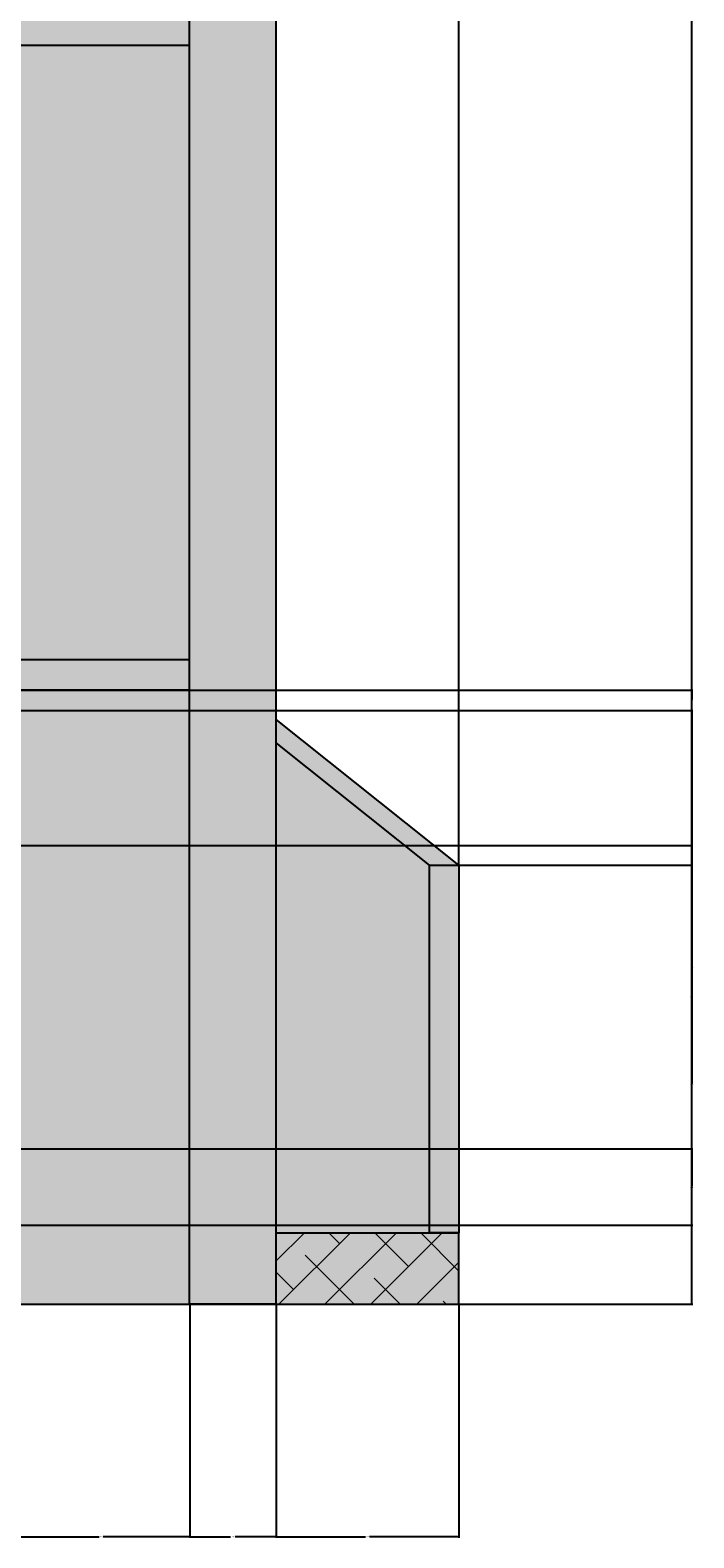
# Model space of a CAD drawing. Units: inches. Extents: x 3024 to 4744, y 1110 to 2100.
# Tile 16 of 29: x 3657 to 3787, y 1110 to 1405. Entities that reach past the tile are written whole.
import ezdxf

# ---------------------------------------------------------------- set-up
doc = ezdxf.new("R2010")
doc.units = ezdxf.units.IN
for name, color, linetype, lineweight in [('A-ANNO-DIMS', 2, 'Continuous', 18), ('A-ELEV', 7, 'Continuous', 25), ('A-ELEV-PATT', 252, 'Continuous', 13)]:
    doc.layers.add(name, color=color, linetype=linetype, lineweight=lineweight)
doc.styles.get("Standard").update_dxf_attribs({"font": 'arial.ttf'})
doc.dimstyles.get("Standard").update_dxf_attribs({"dimtxt": 0.18, "dimasz": 0.18, "dimexe": 0.18, "dimexo": 0.0625, "dimgap": 0.09, "dimtad": 0, "dimtih": 1, "dimtoh": 1, "dimdec": 1, "dimzin": 0, "dimdsep": 46, "dimlunit": 3, "dimtxsty": 'Standard', "dimcen": 0.09, "dimadec": 0, "dimazin": 0, "dimtfac": 1, "dimtdec": 1, "dimtofl": 0, "dimtmove": 0, "dimatfit": 3, "dimfxl": 1, "dimtolj": 1, "dimtzin": 0, "dimarcsym": 0})

# ---------------------------------------------------------------- blocks, each defined once
blk = doc.blocks.new('*D61')
at = {"layer": 'A-ANNO-DIMS', "color": 0, "lineweight": -2, "transparency": 16777216}
for p, q in [((3654.04, 1155.55), (3654.04, 1109.93)), ((3688.56, 1155.55), (3688.56, 1109.93)), ((3654.22, 1110.11), (3670.91, 1110.11)), ((3688.38, 1110.11), (3671.69, 1110.11))]:
    blk.add_line(p, q, dxfattribs=at)
at = {"layer": 'A-ANNO-DIMS', "color": 0, "transparency": 16777216}
for points in [[(3654.22, 1110.14), (3654.22, 1110.08), (3654.04, 1110.11)], [(3688.38, 1110.14), (3688.38, 1110.08), (3688.56, 1110.11)]]:
    blk.add_solid(points, dxfattribs=at)
at = {"layer": 'Defpoints', "color": 0, "transparency": 16777216}
for p in [(3654.04, 1155.61), (3688.56, 1155.61), (3688.56, 1110.11)]:
    blk.add_point(p, dxfattribs=at)
at = {"layer": 'A-ANNO-DIMS', "color": 0, "transparency": 16777216, "insert": (3671.3, 1110.11), "char_height": 0.18, "attachment_point": 5}
blk.add_mtext('\\A1;34.52', dxfattribs=at)
blk = doc.blocks.new('*D62')
at = {"layer": 'A-ANNO-DIMS', "color": 0, "lineweight": -2, "transparency": 16777216}
for p, q in [((3688.56, 1155.55), (3688.56, 1109.93)), ((3705.47, 1155.55), (3705.47, 1109.93)), ((3688.74, 1110.11), (3696.56, 1110.11)), ((3705.29, 1110.11), (3697.47, 1110.11))]:
    blk.add_line(p, q, dxfattribs=at)
at = {"layer": 'A-ANNO-DIMS', "color": 0, "transparency": 16777216}
for points in [[(3688.74, 1110.14), (3688.74, 1110.08), (3688.56, 1110.11)], [(3705.29, 1110.14), (3705.29, 1110.08), (3705.47, 1110.11)]]:
    blk.add_solid(points, dxfattribs=at)
at = {"layer": 'Defpoints', "color": 0, "transparency": 16777216}
for p in [(3688.56, 1155.61), (3705.47, 1155.61), (3705.47, 1110.11)]:
    blk.add_point(p, dxfattribs=at)
at = {"layer": 'A-ANNO-DIMS', "color": 0, "transparency": 16777216, "insert": (3697.02, 1110.11), "char_height": 0.18, "attachment_point": 5}
blk.add_mtext('\\A1;16.913', dxfattribs=at)
blk = doc.blocks.new('*D63')
at = {"layer": 'A-ANNO-DIMS', "color": 0, "lineweight": -2, "transparency": 16777216}
for p, q in [((3705.47, 1155.55), (3705.47, 1109.93)), ((3741.15, 1155.55), (3741.15, 1109.93)), ((3705.65, 1110.11), (3722.92, 1110.11)), ((3740.97, 1110.11), (3723.71, 1110.11))]:
    blk.add_line(p, q, dxfattribs=at)
at = {"layer": 'A-ANNO-DIMS', "color": 0, "transparency": 16777216}
for points in [[(3705.65, 1110.14), (3705.65, 1110.08), (3705.47, 1110.11)], [(3740.97, 1110.14), (3740.97, 1110.08), (3741.15, 1110.11)]]:
    blk.add_solid(points, dxfattribs=at)
at = {"layer": 'Defpoints', "color": 0, "transparency": 16777216}
for p in [(3705.47, 1155.61), (3741.15, 1155.61), (3741.15, 1110.11)]:
    blk.add_point(p, dxfattribs=at)
at = {"layer": 'A-ANNO-DIMS', "color": 0, "transparency": 16777216, "insert": (3723.31, 1110.11), "char_height": 0.18, "attachment_point": 5}
blk.add_mtext('\\A1;35.68', dxfattribs=at)
blk = doc.blocks.new('*D64')
at = {"layer": 'A-ANNO-DIMS', "color": 0, "lineweight": -2, "transparency": 16777216}
for p, q in [((3069.79, 1241.5), (3069.79, 2100.44)), ((3069.97, 2100.26), (3405.08, 2100.26)), ((3740.97, 2100.26), (3405.87, 2100.26)), ((3741.15, 1241.5), (3741.15, 2100.44))]:
    blk.add_line(p, q, dxfattribs=at)
at = {"layer": 'A-ANNO-DIMS', "color": 0, "transparency": 16777216}
for points in [[(3069.97, 2100.29), (3069.97, 2100.23), (3069.79, 2100.26)], [(3740.97, 2100.29), (3740.97, 2100.23), (3741.15, 2100.26)]]:
    blk.add_solid(points, dxfattribs=at)
at = {"layer": 'Defpoints', "color": 0, "transparency": 16777216}
for p in [(3741.15, 2100.26), (3069.79, 1241.43), (3741.15, 1241.43)]:
    blk.add_point(p, dxfattribs=at)
at = {"layer": 'A-ANNO-DIMS', "color": 0, "transparency": 16777216, "insert": (3405.47, 2100.26), "char_height": 0.18, "attachment_point": 5}
blk.add_mtext('\\A1;671.4', dxfattribs=at)
blk = doc.blocks.new('*D75')
at = {"layer": 'A-ANNO-DIMS', "color": 0, "lineweight": -2, "transparency": 16777216}
for p, q in [((3491.89, 2054.76), (3786.83, 2054.76)), ((3786.65, 2054.58), (3786.65, 1605.37)), ((3786.65, 1155.79), (3786.65, 1605)), ((3741.21, 1155.61), (3786.83, 1155.61))]:
    blk.add_line(p, q, dxfattribs=at)
at = {"layer": 'A-ANNO-DIMS', "color": 0, "transparency": 16777216}
for points in [[(3786.62, 2054.58), (3786.68, 2054.58), (3786.65, 2054.76)], [(3786.62, 1155.79), (3786.68, 1155.79), (3786.65, 1155.61)]]:
    blk.add_solid(points, dxfattribs=at)
at = {"layer": 'Defpoints', "color": 0, "transparency": 16777216}
for p in [(3491.83, 2054.76), (3786.65, 2054.76), (3741.15, 1155.61)]:
    blk.add_point(p, dxfattribs=at)
at = {"layer": 'A-ANNO-DIMS', "color": 0, "transparency": 16777216, "insert": (3786.65, 1605.18), "char_height": 0.18, "attachment_point": 5}
blk.add_mtext('\\A1;899.1', dxfattribs=at)
blk = doc.blocks.new('*D79')
at = {"layer": 'A-ANNO-DIMS', "color": 0, "lineweight": -2, "transparency": 16777216}
for p, q in [((3741.21, 1241.43), (3786.83, 1241.43)), ((3786.65, 1241.25), (3786.65, 1198.7)), ((3786.65, 1155.79), (3786.65, 1198.34)), ((3741.21, 1155.61), (3786.83, 1155.61))]:
    blk.add_line(p, q, dxfattribs=at)
at = {"layer": 'A-ANNO-DIMS', "color": 0, "transparency": 16777216}
for points in [[(3786.62, 1241.25), (3786.68, 1241.25), (3786.65, 1241.43)], [(3786.62, 1155.79), (3786.68, 1155.79), (3786.65, 1155.61)]]:
    blk.add_solid(points, dxfattribs=at)
at = {"layer": 'Defpoints', "color": 0, "transparency": 16777216}
for p in [(3741.15, 1241.43), (3786.65, 1241.43), (3741.15, 1155.61)]:
    blk.add_point(p, dxfattribs=at)
at = {"layer": 'A-ANNO-DIMS', "color": 0, "transparency": 16777216, "insert": (3786.65, 1198.52), "char_height": 0.18, "attachment_point": 5}
blk.add_mtext('\\A1;85.82', dxfattribs=at)
blk = doc.blocks.new('*D120')
at = {"layer": 'A-ANNO-DIMS', "color": 0, "lineweight": -2, "transparency": 16777216}
for p, q in [((3270.45, 1271.61), (3786.83, 1271.61)), ((3786.65, 1271.43), (3786.65, 1221.5)), ((3786.65, 1171.2), (3786.65, 1221.14)), ((3274.45, 1171.02), (3786.83, 1171.02))]:
    blk.add_line(p, q, dxfattribs=at)
at = {"layer": 'A-ANNO-DIMS', "color": 0, "transparency": 16777216}
for points in [[(3786.62, 1271.43), (3786.68, 1271.43), (3786.65, 1271.61)], [(3786.62, 1171.2), (3786.68, 1171.2), (3786.65, 1171.02)]]:
    blk.add_solid(points, dxfattribs=at)
at = {"layer": 'Defpoints', "color": 0, "transparency": 16777216}
for p in [(3270.39, 1271.61), (3786.65, 1271.61), (3274.39, 1171.02)]:
    blk.add_point(p, dxfattribs=at)
at = {"layer": 'A-ANNO-DIMS', "color": 0, "transparency": 16777216, "insert": (3786.65, 1221.32), "char_height": 0.18, "attachment_point": 5}
blk.add_mtext('\\A1;100.59', dxfattribs=at)
blk = doc.blocks.new('*D121')
at = {"layer": 'A-ANNO-DIMS', "color": 0, "lineweight": -2, "transparency": 16777216}
for p, q in [((3274.45, 1275.61), (3786.83, 1275.61)), ((3786.65, 1275.43), (3786.65, 1273.79)), ((3786.65, 1271.79), (3786.65, 1273.43)), ((3270.45, 1271.61), (3786.83, 1271.61))]:
    blk.add_line(p, q, dxfattribs=at)
at = {"layer": 'A-ANNO-DIMS', "color": 0, "transparency": 16777216}
for points in [[(3786.62, 1275.43), (3786.68, 1275.43), (3786.65, 1275.61)], [(3786.62, 1271.79), (3786.68, 1271.79), (3786.65, 1271.61)]]:
    blk.add_solid(points, dxfattribs=at)
at = {"layer": 'Defpoints', "color": 0, "transparency": 16777216}
for p in [(3274.39, 1275.61), (3786.65, 1275.61), (3270.39, 1271.61)]:
    blk.add_point(p, dxfattribs=at)
at = {"layer": 'A-ANNO-DIMS', "color": 0, "transparency": 16777216, "insert": (3786.65, 1273.61), "char_height": 0.18, "attachment_point": 5}
blk.add_mtext('\\A1;4.00', dxfattribs=at)
blk = doc.blocks.new('*D122')
at = {"layer": 'A-ANNO-DIMS', "color": 0, "lineweight": -2, "transparency": 16777216}
for p, q in [((3228.45, 1185.95), (3786.83, 1185.95)), ((3786.65, 1185.77), (3786.65, 1178.67)), ((3786.65, 1171.2), (3786.65, 1178.31)), ((3270.45, 1171.02), (3786.83, 1171.02))]:
    blk.add_line(p, q, dxfattribs=at)
at = {"layer": 'A-ANNO-DIMS', "color": 0, "transparency": 16777216}
for points in [[(3786.62, 1185.77), (3786.68, 1185.77), (3786.65, 1185.95)], [(3786.62, 1171.2), (3786.68, 1171.2), (3786.65, 1171.02)]]:
    blk.add_solid(points, dxfattribs=at)
at = {"layer": 'Defpoints', "color": 0, "transparency": 16777216}
for p in [(3228.39, 1185.95), (3270.39, 1171.02), (3786.65, 1171.02)]:
    blk.add_point(p, dxfattribs=at)
at = {"layer": 'A-ANNO-DIMS', "color": 0, "transparency": 16777216, "insert": (3786.65, 1178.49), "char_height": 0.18, "attachment_point": 5}
blk.add_mtext('\\A1;14.928', dxfattribs=at)
blk = doc.blocks.new('*D123')
at = {"layer": 'A-ANNO-DIMS', "color": 0, "lineweight": -2, "transparency": 16777216}
for p, q in [((3228.45, 1245.27), (3786.83, 1245.27)), ((3786.65, 1245.09), (3786.65, 1215.79)), ((3786.65, 1186.13), (3786.65, 1215.43)), ((3228.45, 1185.95), (3786.83, 1185.95))]:
    blk.add_line(p, q, dxfattribs=at)
at = {"layer": 'A-ANNO-DIMS', "color": 0, "transparency": 16777216}
for points in [[(3786.62, 1245.09), (3786.68, 1245.09), (3786.65, 1245.27)], [(3786.62, 1186.13), (3786.68, 1186.13), (3786.65, 1185.95)]]:
    blk.add_solid(points, dxfattribs=at)
at = {"layer": 'Defpoints', "color": 0, "transparency": 16777216}
for p in [(3228.39, 1245.27), (3786.65, 1245.27), (3228.39, 1185.95)]:
    blk.add_point(p, dxfattribs=at)
at = {"layer": 'A-ANNO-DIMS', "color": 0, "transparency": 16777216, "insert": (3786.65, 1215.61), "char_height": 0.18, "attachment_point": 5}
blk.add_mtext('\\A1;59.32', dxfattribs=at)

msp = doc.modelspace()

# ---------------------------------------------------------------- hatches: boundary and pattern name
at = {"layer": 'A-ELEV-PATT'}
h = msp.add_hatch(color=256, dxfattribs=at)
h.dxf.hatch_style = 1
h.paths.add_polyline_path([(3705.4722, 2014.6567), (3688.5588, 2014.6567), (3481.2411, 2014.6567), (3481.2411, 2009.1664), (3688.5588, 2009.1664), (3688.5588, 1155.6112), (3705.4722, 1155.6112), (3705.4722, 1911.6112)])
h = msp.add_hatch(color=256, dxfattribs=at)
h.dxf.hatch_style = 1
h.paths.add_polyline_path([(3154.3287, 1897.4879), (3148.9694, 1897.4879), (3148.9694, 1905.6112), (3105.4722, 1905.6112), (3105.4722, 1785.6112), (3148.9694, 1785.6112), (3148.9694, 1795.0431), (3151.6604, 1795.0431), (3151.6604, 1806.8674), (3154.3287, 1806.8674)])
h.paths.add_polyline_path([(3329.7033, 1905.6112), (3292.6051, 1905.6112), (3292.6051, 1897.4879), (3287.2458, 1897.4879), (3287.2458, 1806.8674), (3288.3759, 1806.8674), (3288.3759, 1795.0431), (3292.6051, 1795.0431), (3292.6051, 1785.6112), (3329.7033, 1785.6112)])
h.paths.add_polyline_path([(3154.3287, 1771.4879), (3148.9694, 1771.4879), (3148.9694, 1779.6112), (3105.4722, 1779.6112), (3105.4722, 1659.6112), (3148.9694, 1659.6112), (3148.9694, 1669.0431), (3151.6604, 1669.0431), (3151.6604, 1680.8674), (3154.3287, 1680.8674)])
h.paths.add_polyline_path([(3329.7033, 1779.6112), (3292.6051, 1779.6112), (3292.6051, 1771.4879), (3287.2458, 1771.4879), (3287.2458, 1680.8674), (3288.3759, 1680.8674), (3288.3759, 1669.0431), (3292.6051, 1669.0431), (3292.6051, 1659.6112), (3329.7033, 1659.6112)])
h.paths.add_polyline_path([(3154.3287, 1645.4879), (3148.9694, 1645.4879), (3148.9694, 1653.6112), (3105.4722, 1653.6112), (3105.4722, 1533.6112), (3148.9694, 1533.6112), (3148.9694, 1543.0431), (3151.6604, 1543.0431), (3151.6604, 1554.8674), (3154.3287, 1554.8674)])
h.paths.add_polyline_path([(3329.7033, 1653.6112), (3292.6051, 1653.6112), (3292.6051, 1645.4879), (3287.2458, 1645.4879), (3287.2458, 1554.8674), (3288.3759, 1554.8674), (3288.3759, 1543.0431), (3292.6051, 1543.0431), (3292.6051, 1533.6112), (3329.7033, 1533.6112)])
h.paths.add_polyline_path([(3329.7033, 1527.6112), (3292.6051, 1527.6112), (3292.6051, 1519.4879), (3287.2458, 1519.4879), (3287.2458, 1428.8674), (3288.3759, 1428.8674), (3288.3759, 1417.0431), (3292.6051, 1417.0431), (3292.6051, 1407.6112), (3329.7033, 1407.6112)])
h.paths.add_polyline_path([(3329.7033, 1401.6112), (3292.6051, 1401.6112), (3292.6051, 1393.4879), (3287.2458, 1393.4879), (3287.2458, 1302.8674), (3288.3759, 1302.8674), (3288.3759, 1291.0431), (3292.6051, 1291.0431), (3292.6051, 1281.6112), (3329.7033, 1281.6112)])
h.paths.add_polyline_path([(3154.3287, 1393.4879), (3148.9694, 1393.4879), (3148.9694, 1401.6112), (3105.4722, 1401.6112), (3105.4722, 1281.6112), (3148.9694, 1281.6112), (3148.9694, 1291.0431), (3151.6604, 1291.0431), (3151.6604, 1302.8674), (3154.3287, 1302.8674)])
h.paths.add_polyline_path([(3154.3287, 1519.4879), (3148.9694, 1519.4879), (3148.9694, 1527.6112), (3105.4722, 1527.6112), (3105.4722, 1407.6112), (3148.9694, 1407.6112), (3148.9694, 1417.0431), (3151.6604, 1417.0431), (3151.6604, 1428.8674), (3154.3287, 1428.8674)])
h.paths.add_polyline_path([(3515.7606, 1897.4879), (3510.4013, 1897.4879), (3510.4013, 1905.6112), (3481.2411, 1905.6112), (3481.2411, 1785.6112), (3510.4013, 1785.6112), (3510.4013, 1795.0431), (3513.0923, 1795.0431), (3513.0923, 1806.8674), (3515.7606, 1806.8674)])
h.paths.add_polyline_path([(3688.5588, 1905.6112), (3654.037, 1905.6112), (3654.037, 1897.4879), (3648.6777, 1897.4879), (3648.6777, 1806.8674), (3649.8078, 1806.8674), (3649.8078, 1795.0431), (3654.037, 1795.0431), (3654.037, 1785.6112), (3688.5588, 1785.6112)])
h.paths.add_polyline_path([(3515.7606, 1771.4879), (3510.4013, 1771.4879), (3510.4013, 1779.6112), (3481.2411, 1779.6112), (3481.2411, 1659.6112), (3510.4013, 1659.6112), (3510.4013, 1669.0431), (3513.0923, 1669.0431), (3513.0923, 1680.8674), (3515.7606, 1680.8674)])
h.paths.add_polyline_path([(3688.5588, 1779.6112), (3654.037, 1779.6112), (3654.037, 1771.4879), (3648.6777, 1771.4879), (3648.6777, 1680.8674), (3649.8078, 1680.8674), (3649.8078, 1669.0431), (3654.037, 1669.0431), (3654.037, 1659.6112), (3688.5588, 1659.6112)])
h.paths.add_polyline_path([(3515.7606, 1645.4879), (3510.4013, 1645.4879), (3510.4013, 1653.6112), (3481.2411, 1653.6112), (3481.2411, 1533.6112), (3510.4013, 1533.6112), (3510.4013, 1543.0431), (3513.0923, 1543.0431), (3513.0923, 1554.8674), (3515.7606, 1554.8674)])
h.paths.add_polyline_path([(3688.5588, 1653.6112), (3654.037, 1653.6112), (3654.037, 1645.4879), (3648.6777, 1645.4879), (3648.6777, 1554.8674), (3649.8078, 1554.8674), (3649.8078, 1543.0431), (3654.037, 1543.0431), (3654.037, 1533.6112), (3688.5588, 1533.6112)])
h.paths.add_polyline_path([(3515.7606, 1519.4879), (3510.4013, 1519.4879), (3510.4013, 1527.6112), (3481.2411, 1527.6112), (3481.2411, 1407.6112), (3510.4013, 1407.6112), (3510.4013, 1417.0431), (3513.0923, 1417.0431), (3513.0923, 1428.8674), (3515.7606, 1428.8674)])
h.paths.add_polyline_path([(3688.5588, 1527.6112), (3654.037, 1527.6112), (3654.037, 1519.4879), (3648.6777, 1519.4879), (3648.6777, 1428.8674), (3649.8078, 1428.8674), (3649.8078, 1417.0431), (3654.037, 1417.0431), (3654.037, 1407.6112), (3688.5588, 1407.6112)])
h.paths.add_polyline_path([(3515.7606, 1393.4879), (3510.4013, 1393.4879), (3510.4013, 1401.6112), (3481.2411, 1401.6112), (3481.2411, 1281.6112), (3510.4013, 1281.6112), (3510.4013, 1291.0431), (3513.0923, 1291.0431), (3513.0923, 1302.8674), (3515.7606, 1302.8674)])
h.paths.add_polyline_path([(3688.5588, 1401.6112), (3654.037, 1401.6112), (3654.037, 1393.4879), (3648.6777, 1393.4879), (3648.6777, 1302.8674), (3649.8078, 1302.8674), (3649.8078, 1291.0431), (3654.037, 1291.0431), (3654.037, 1281.6112), (3688.5588, 1281.6112)])
h.paths.add_polyline_path([(3515.7606, 1267.4879), (3510.4013, 1267.4879), (3510.4013, 1275.6112), (3481.2411, 1275.6112), (3481.2411, 1155.6112), (3510.4013, 1155.6112), (3510.4013, 1165.0431), (3513.0923, 1165.0431), (3513.0923, 1176.8674), (3515.7606, 1176.8674)])
h.paths.add_polyline_path([(3688.5588, 1275.6112), (3654.037, 1275.6112), (3654.037, 1267.4879), (3648.6777, 1267.4879), (3648.6777, 1176.8674), (3649.8078, 1176.8674), (3649.8078, 1165.0431), (3654.037, 1165.0431), (3654.037, 1155.6112), (3688.5588, 1155.6112)])
h.paths.add_polyline_path([(3112.3838, 1275.6112), (3105.4722, 1275.6112), (3105.4722, 1171.0239), (3112.3838, 1171.0239)])
h = msp.add_hatch(color=256, dxfattribs=at)
h.dxf.hatch_style = 1
h.paths.add_polyline_path([(3688.5588, 1785.6112), (3481.2411, 1785.6112), (3481.2411, 1779.6112), (3688.5588, 1779.6112)])
h.paths.add_polyline_path([(3688.5588, 1659.6112), (3481.2411, 1659.6112), (3481.2411, 1653.6112), (3688.5588, 1653.6112)])
h.paths.add_polyline_path([(3688.5588, 1533.6112), (3481.2411, 1533.6112), (3481.2411, 1527.6112), (3688.5588, 1527.6112)])
h.paths.add_polyline_path([(3688.5588, 1407.6112), (3481.2411, 1407.6112), (3481.2411, 1401.6112), (3688.5588, 1401.6112)])
h.paths.add_polyline_path([(3688.5588, 1281.6112), (3481.2411, 1281.6112), (3481.2411, 1275.6112), (3688.5588, 1275.6112)])
h = msp.add_hatch(color=256, dxfattribs=at)
h.dxf.hatch_style = 1
h.paths.add_polyline_path([(3329.7033, 1171.0239), (3256.7794, 1171.0239, -0.21182003), (3255.8005, 1171.0239), (3249.6327, 1171.0239, -0.21182003), (3248.6539, 1171.0239), (3195.8947, 1171.0239, -0.21182003), (3194.9159, 1171.0239), (3188.7481, 1171.0239, -0.21182003), (3187.7692, 1171.0239), (3118.1176, 1171.0239), (3115.5754, 1168.0828), (3115.5754, 1155.6112), (3329.7033, 1155.6112)])
h.paths.add_polyline_path([(3101.9647, 1168.0828), (3103.2358, 1169.5534), (3069.7937, 1169.5534), (3069.7937, 1155.6112), (3101.9647, 1155.6112)])
h.paths.add_polyline_path([(3115.5754, 1168.0828), (3101.9647, 1168.0828), (3101.9647, 1155.6112), (3105.4722, 1155.6112), (3115.5754, 1155.6112)])
h.paths.add_polyline_path([(3118.1176, 1171.0239), (3104.5069, 1171.0239), (3101.9647, 1168.0828), (3115.5754, 1168.0828)])
h.paths.add_polyline_path([(3105.4722, 1265.3254), (3075.5369, 1241.4341), (3075.5369, 1169.5534), (3103.2358, 1169.5534), (3104.5069, 1171.0239), (3105.4722, 1171.0239)])
h.paths.add_polyline_path([(3105.4722, 1265.3254), (3105.4722, 1269.9091), (3069.7937, 1241.4341), (3075.5369, 1241.4341)])
h.paths.add_polyline_path([(3075.5369, 1241.4341), (3069.7937, 1241.4341), (3069.7937, 1169.5534), (3075.5369, 1169.5534)])
h.paths.add_polyline_path([(3735.4075, 1241.4341), (3705.4722, 1265.3254), (3705.4722, 1169.5534), (3735.4075, 1169.5534)])
h.paths.add_polyline_path([(3705.4722, 1269.9091), (3705.4722, 1265.3254), (3735.4075, 1241.4341), (3741.1507, 1241.4341)])
h.paths.add_polyline_path([(3741.1507, 1241.4341), (3735.4075, 1241.4341), (3735.4075, 1169.5534), (3741.1507, 1169.5534)])
h.paths.add_polyline_path([(3741.1507, 1169.5534), (3735.4075, 1169.5534), (3705.4722, 1169.5534), (3705.4722, 1155.6112), (3741.1507, 1155.6112)])
h = msp.add_hatch(dxfattribs=at)
h.set_pattern_fill('AR-B816', color=256, scale=0.01)
h.paths.add_polyline_path([(3105.4722, 1265.3254), (3075.5369, 1241.4341), (3075.5369, 1169.5534), (3103.2358, 1169.5534), (3104.5069, 1171.0239), (3105.4722, 1171.0239)])
h.paths.add_polyline_path([(3105.4722, 1265.3254), (3105.4722, 1269.9091), (3069.7937, 1241.4341), (3075.5369, 1241.4341)])
h.paths.add_polyline_path([(3075.5369, 1241.4341), (3069.7937, 1241.4341), (3069.7937, 1169.5534), (3075.5369, 1169.5534)])
h.paths.add_polyline_path([(3735.4075, 1241.4341), (3705.4722, 1265.3254), (3705.4722, 1169.5534), (3735.4075, 1169.5534)])
h.paths.add_polyline_path([(3705.4722, 1269.9091), (3705.4722, 1265.3254), (3735.4075, 1241.4341), (3741.1507, 1241.4341)])
h.paths.add_polyline_path([(3741.1507, 1241.4341), (3735.4075, 1241.4341), (3735.4075, 1169.5534), (3741.1507, 1169.5534)])
h = msp.add_hatch(dxfattribs=at)
h.set_pattern_fill('ANSI38', color=256, scale=2)
h.paths.add_polyline_path([(3101.9647, 1168.0828), (3103.2358, 1169.5534), (3069.7937, 1169.5534), (3069.7937, 1155.6112), (3101.9647, 1155.6112)])
h.paths.add_polyline_path([(3115.5754, 1168.0828), (3101.9647, 1168.0828), (3101.9647, 1155.6112), (3105.4722, 1155.6112), (3115.5754, 1155.6112)])
h.paths.add_polyline_path([(3118.1176, 1171.0239), (3104.5069, 1171.0239), (3101.9647, 1168.0828), (3115.5754, 1168.0828)])
h.paths.add_polyline_path([(3329.7033, 1171.0239), (3256.7794, 1171.0239, -0.21182003), (3255.8005, 1171.0239), (3249.6327, 1171.0239, -0.21182003), (3248.6539, 1171.0239), (3195.8947, 1171.0239, -0.21182003), (3194.9159, 1171.0239), (3188.7481, 1171.0239, -0.21182003), (3187.7692, 1171.0239), (3118.1176, 1171.0239), (3115.5754, 1168.0828), (3115.5754, 1155.6112), (3329.7033, 1155.6112)])
h.paths.add_polyline_path([(3741.1507, 1169.5534), (3735.4075, 1169.5534), (3705.4722, 1169.5534), (3705.4722, 1155.6112), (3741.1507, 1155.6112)])

# ---------------------------------------------------------------- linework, layer by layer
at = {"layer": 'A-ELEV'}
for p, q in [((3705.4722, 1155.6112), (3705.4722, 1911.6112)), ((3705.4722, 1155.6112), (3705.4722, 1911.6112)), ((3688.5588, 1401.6112), (3481.2411, 1401.6112)), ((3688.5588, 1401.6112), (3481.2411, 1401.6112)), ((3481.2411, 1281.6112), (3688.5588, 1281.6112)), ((3481.2411, 1281.6112), (3688.5588, 1281.6112)), ((3688.5588, 1275.6112), (3481.2411, 1275.6112)), ((3688.5588, 1275.6112), (3481.2411, 1275.6112)), ((3741.1507, 1241.4341), (3705.4722, 1269.9091)), ((3741.1507, 1241.4341), (3705.4722, 1269.9091)), ((3735.4075, 1241.4341), (3705.4722, 1265.3254)), ((3735.4075, 1241.4341), (3705.4722, 1265.3254)), ((3705.4722, 1169.5534), (3741.1507, 1169.5534)), ((3705.4722, 1169.5534), (3741.1507, 1169.5534)), ((3741.1507, 1155.6112), (3741.1507, 1169.5534)), ((3741.1507, 1155.6112), (3741.1507, 1169.5534)), ((3105.4722, 1155.6112), (3705.4722, 1155.6112)), ((3105.4722, 1155.6112), (3705.4722, 1155.6112)), ((3705.4722, 1155.6112), (3741.1507, 1155.6112)), ((3705.4722, 1155.6112), (3741.1507, 1155.6112))]:
    msp.add_line(p, q, dxfattribs=at)
for points in [[(3705.4722, 1155.6112), (3688.5588, 1155.6112), (3688.5588, 2014.6567), (3705.4722, 2014.6567), (3705.4722, 1905.6112)], [(3705.4722, 1155.6112), (3688.5588, 1155.6112), (3688.5588, 2009.1664)]]:
    msp.add_lwpolyline(points, dxfattribs=at)
msp.add_lwpolyline([(3741.1507, 1169.5534), (3735.4075, 1169.5534), (3735.4075, 1241.4341), (3741.1507, 1241.4341)], close=True, dxfattribs=at)
msp.add_lwpolyline([(3741.1507, 1169.5534), (3735.4075, 1169.5534), (3735.4075, 1241.4341), (3741.1507, 1241.4341)], close=True, dxfattribs=at)

# ---------------------------------------------------------------- dimensions: what is measured, and where the dimension line sits
at = {"layer": 'A-ANNO-DIMS'}
for base, p1, p2, override, picture, middle in [((3741.1507, 2100.2584), (3069.7937, 1241.4341), (3741.1507, 1241.4341), {"dimdec": 1, "dimlfac": 1, "dimrnd": 0, "dimzin": 0, "dimdsep": 46, "dimlunit": 2}, '*D64', (3405.4722, 2100.2584)), ((3688.5588, 1110.1112), (3654.037, 1155.6112), (3688.5588, 1155.6112), {"dimdec": 2, "dimlfac": 1, "dimrnd": 0, "dimzin": 0, "dimdsep": 46, "dimlunit": 2}, '*D61', (3671.2979, 1110.1112)), ((3705.4722, 1110.1112), (3688.5588, 1155.6112), (3705.4722, 1155.6112), {"dimdec": 3, "dimlfac": 1, "dimrnd": 0, "dimzin": 0, "dimdsep": 46, "dimlunit": 2}, '*D62', (3697.0155, 1110.1112)), ((3741.1507, 1110.1112), (3705.4722, 1155.6112), (3741.1507, 1155.6112), {"dimdec": 2, "dimlfac": 1, "dimrnd": 0, "dimzin": 0, "dimdsep": 46, "dimlunit": 2}, '*D63', (3723.3115, 1110.1112))]:
    dim = msp.add_linear_dim(base=base, p1=p1, p2=p2, dimstyle='Standard', override=override, dxfattribs=at)
    dim.commit()
    dim.dimension.update_dxf_attribs({"geometry": picture, "text_midpoint": middle})
for base, p1, p2, override, picture, middle in [((3786.6507, 2054.7584), (3741.1507, 1155.6112), (3491.8271, 2054.7584), {"dimdec": 1, "dimlfac": 1, "dimrnd": 0, "dimzin": 0, "dimdsep": 46, "dimlunit": 2}, '*D75', (3786.6507, 1605.1848)), ((3786.6507, 1275.6112), (3270.3877, 1271.6112), (3274.3877, 1275.6112), {"dimdec": 2, "dimlfac": 1, "dimrnd": 0, "dimzin": 0, "dimdsep": 46, "dimlunit": 2}, '*D121', (3786.6507, 1273.6112)), ((3786.6507, 1271.6112), (3274.3877, 1171.0239), (3270.3877, 1271.6112), {"dimdec": 2, "dimlfac": 1, "dimrnd": 0, "dimzin": 0, "dimdsep": 46, "dimlunit": 2}, '*D120', (3786.6507, 1221.3176)), ((3786.6507, 1245.2708), (3228.3856, 1185.9515), (3228.3856, 1245.2708), {"dimdec": 2, "dimlfac": 1, "dimrnd": 0, "dimzin": 0, "dimdsep": 46, "dimlunit": 2}, '*D123', (3786.6507, 1215.6112)), ((3786.6507, 1241.4341), (3741.1507, 1155.6112), (3741.1507, 1241.4341), {"dimdec": 2, "dimlfac": 1, "dimrnd": 0, "dimzin": 0, "dimdsep": 46, "dimlunit": 2}, '*D79', (3786.6507, 1198.5226)), ((3786.6507, 1171.0239), (3228.3856, 1185.9515), (3270.3877, 1171.0239), {"dimdec": 3, "dimlfac": 1, "dimrnd": 0, "dimzin": 0, "dimdsep": 46, "dimlunit": 2}, '*D122', (3786.6507, 1178.4877))]:
    dim = msp.add_linear_dim(base=base, p1=p1, p2=p2, angle=90, dimstyle='Standard', override=override, dxfattribs=at)
    dim.commit()
    dim.dimension.update_dxf_attribs({"geometry": picture, "text_midpoint": middle})

doc.saveas('drawing.dxf')
